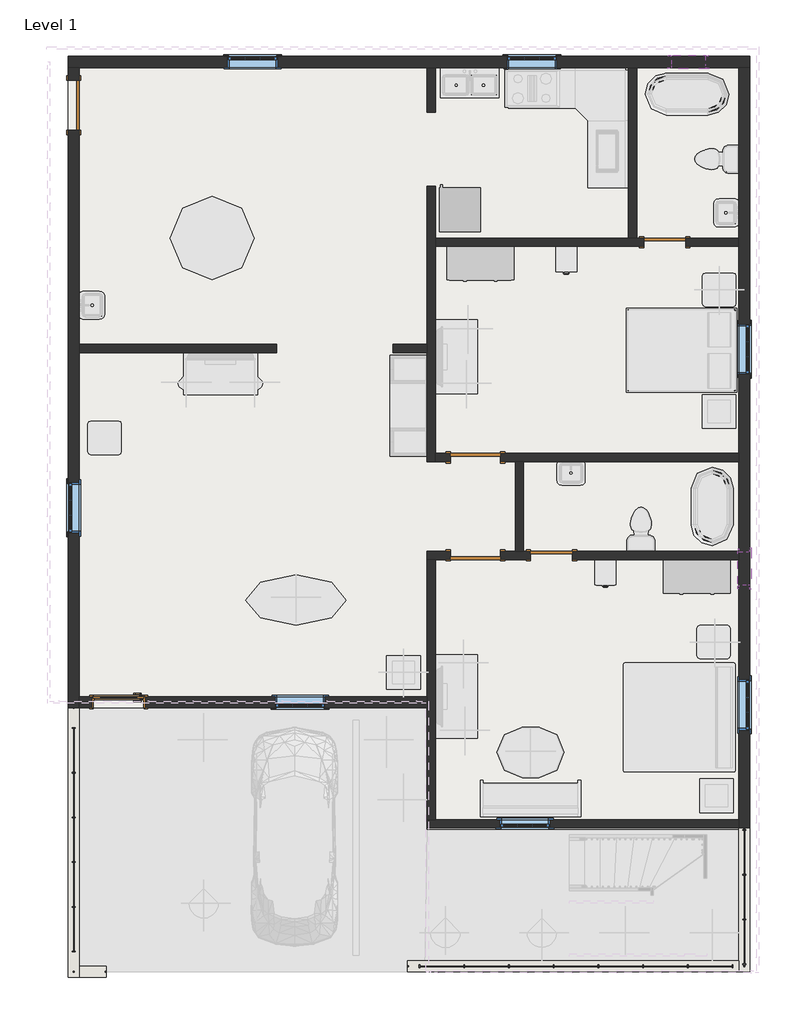
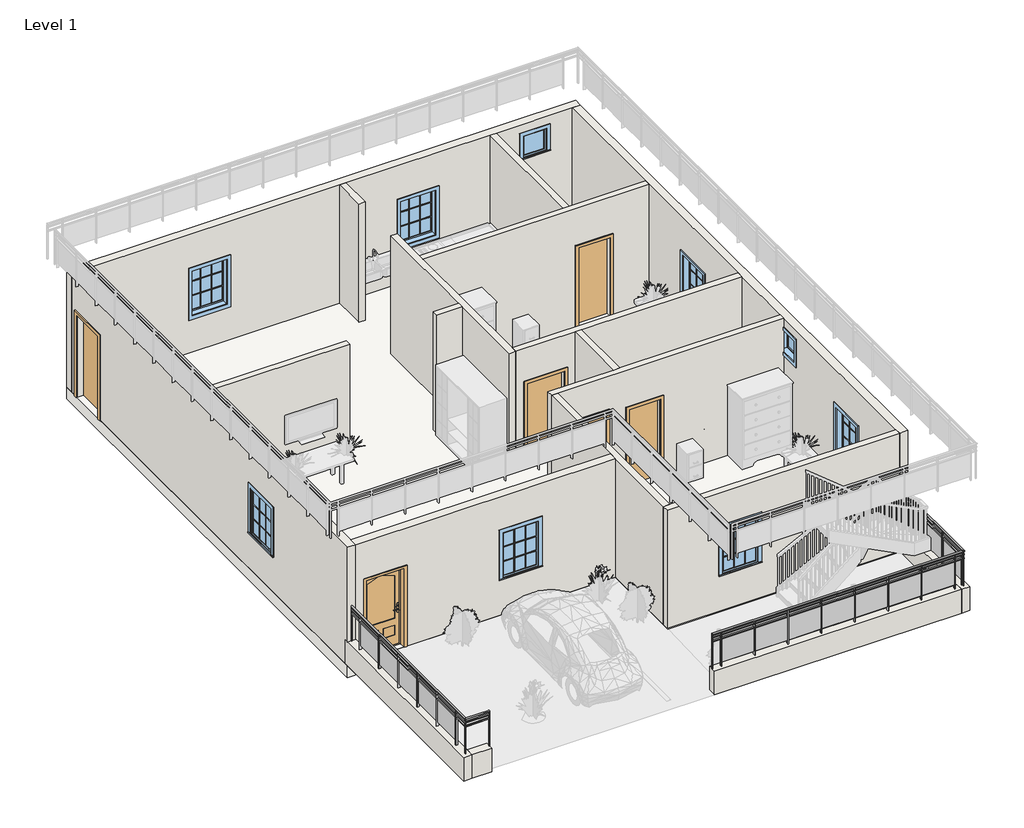
# One storey, part 1 of 5: 19 walls, 9 windows, 6 doors, 2 railings, 1 slab.
"""IFC4 building model written with IfcOpenShell, lengths in millimetres."""

from ifc_helpers import new_model, si_unit, frame, origin, origin_with_axes, place, context, project, spatial, polyline, circle_curve, ellipse_curve, outline, extrude, faceted_brep, transform, mapped, element, save
from ifc_brep_helpers import plane_surface, cylinder_surface, advanced_brep
from components import door_1768e003, door_255cab33, door_719f80de, door_16372e1c, door_686f89d2, window_29c06734, window_5c190c7e, window_e41d21a6

model = new_model("IFC4")

# Units and contexts
model_context = context("Model", 3, world=origin())
ifc_project = project(units=[si_unit("LENGTHUNIT", "METRE", prefix="MILLI")], contexts=[model_context])

# Site, building, storey
site = spatial("IfcSite", under=ifc_project)
building = spatial("IfcBuilding", under=site)
storey = spatial("IfcBuildingStorey", under=building, Name="Level 1", Elevation=0.0)

# Doors
placement = place(None, origin())
door_shape = door_1768e003(model_context)
element("IfcDoor", 1, ObjectType="36\" x 80\"", at=placement, inside=storey, context=model_context, shape_type="MappedRepresentation", body=[
    mapped(door_shape, transform((-11404.4241134, 2269.2383056, 0.0), x_axis=(1.0, 0.0, 0.0), y_axis=(0.0, 1.0, 0.0), z_axis=(0.0, 0.0, 1.0))),
])
door_2_shape = door_255cab33(model_context)
element("IfcDoor", 2, ObjectType="Single-Flush : 30\" x 80\"", at=placement, inside=storey, context=model_context, shape_type="MappedRepresentation", body=[
    mapped(door_2_shape, transform((-3530.4241134, 4933.0633056, 0.0), x_axis=(-1.0, 0.0, 0.0), y_axis=(0.0, -1.0, 0.0), z_axis=(0.0, 0.0, 1.0))),
])
element("IfcDoor", 3, ObjectType="Single-Flush : 30\" x 80\"", at=placement, inside=storey, context=model_context, shape_type="MappedRepresentation", body=[
    mapped(door_2_shape, transform((-1473.0241134, 10622.6633056, 0.0), x_axis=(-1.0, 0.0, 0.0), y_axis=(0.0, -1.0, 0.0), z_axis=(0.0, 0.0, 1.0))),
])
door_3_shape = door_719f80de(model_context)
element("IfcDoor", 4, ObjectType="Single-Flush : 36\" x 84\"", at=placement, inside=storey, context=model_context, shape_type="MappedRepresentation", body=[
    mapped(door_3_shape, transform((-12217.2241134, 13111.8633056, 0.0), x_axis=(0.0, 1.0, 0.0), y_axis=(-1.0, 0.0, 0.0), z_axis=(0.0, 0.0, 1.0))),
])
door_4_shape = door_16372e1c(model_context)
element("IfcDoor", 5, ObjectType="Single-Flush : 36\" x 84\"", at=placement, inside=storey, context=model_context, shape_type="MappedRepresentation", body=[
    mapped(door_4_shape, transform((-4914.7241134, 4933.0633056, 0.0), x_axis=(-1.0, 0.0, 0.0), y_axis=(0.0, -1.0, 0.0), z_axis=(0.0, 0.0, 1.0))),
])
door_5_shape = door_686f89d2(model_context)
element("IfcDoor", 6, ObjectType="Single-Flush : 36\" x 84\"", at=placement, inside=storey, context=model_context, shape_type="MappedRepresentation", body=[
    mapped(door_5_shape, transform((-4914.7241134, 6711.0633056, 0.0), x_axis=(-1.0, 0.0, 0.0), y_axis=(0.0, -1.0, 0.0), z_axis=(0.0, 0.0, 1.0))),
])

# Railings
element("IfcRailing", 7, ObjectType="Glass Panel - Bottom Fill", at=placement, inside=storey, context=model_context, shape_type="SolidModel", body=[
    advanced_brep(
    [(-12236.2741134, 2164.4633056, 1504.95), (-12198.1741134, 2164.4633056, 1504.95), (-11633.0241134, -2655.1866944, 1504.95), (-11633.0241134, -2617.0866944, 1504.95), (-12236.2741134, -2655.1866944, 1504.95), (-12198.1741134, -2617.0866944, 1504.95)],
    [
        (0, 1, circle_curve(frame((-12217.2241134, 2164.4633056, 1504.95), z_axis=(0.0, 1.0, 0.0), x_axis=(1.0, 0.0, 0.0)), 19.05)),
        (1, 0, circle_curve(frame((-12217.2241134, 2164.4633056, 1504.95), z_axis=(0.0, 1.0, 0.0), x_axis=(1.0, 0.0, 0.0)), 19.05)),
        (2, 3, circle_curve(frame((-11633.0241134, -2636.1366944, 1504.95), z_axis=(1.0, 0.0, 0.0), x_axis=(0.0, 1.0, 0.0)), 19.05)),
        (3, 2, circle_curve(frame((-11633.0241134, -2636.1366944, 1504.95), z_axis=(1.0, 0.0, 0.0), x_axis=(0.0, 1.0, 0.0)), 19.05)),
        (0, 4),
        (4, 5, ellipse_curve(frame((-12217.2241134, -2636.1366944, 1504.95), z_axis=(-0.707106781186546, 0.7071067811865491, 0.0), x_axis=(0.7071067811865492, 0.7071067811865458, 0.0)), 26.9407684, 19.05)),
        (5, 1),
        (5, 4, ellipse_curve(frame((-12217.2241134, -2636.1366944, 1504.95), z_axis=(-0.707106781186546, 0.7071067811865491, 0.0), x_axis=(0.7071067811865492, 0.7071067811865458, 0.0)), 26.9407684, 19.05)),
        (4, 2),
        (3, 5),
    ],
    [
        plane_surface(frame((-12217.2241134, 2164.4633056, 1524.0), z_axis=(0.0, 1.0, 0.0), x_axis=(0.0, 0.0, -1.0))),
        plane_surface(frame((-11633.0241134, -2636.1366944, 1524.0), z_axis=(1.0, 0.0, 0.0), x_axis=(0.0, 1.0, 0.0))),
        cylinder_surface(frame((-12217.2241134, 2164.4633056, 1504.95), z_axis=(0.0, 1.0, 0.0), x_axis=(1.0, 0.0, 0.0)), 19.05),
        cylinder_surface(frame((-12217.2241134, -2636.1366944, 1504.95), z_axis=(-1.0, 0.0, 0.0), x_axis=(0.0, 1.0, 0.0)), 19.05),
    ],
    [
        (0, [[1, 2]]),
        (1, [[3, 4]]),
        (2, [[-1, 5, 6, 7]]),
        (2, [[-2, -7, 8, -5]]),
        (3, [[-6, 9, -4, 10]]),
        (3, [[-8, -10, -3, -9]]),
    ],
),
    faceted_brep([(-12229.9241134, 2164.4633056, 1435.1), (-12204.5241134, 2164.4633056, 1435.1), (-12204.5241134, 2164.4633056, 1409.7), (-12229.9241134, 2164.4633056, 1409.7), (-12229.9241134, -2648.8366944, 1435.1), (-12204.5241134, -2623.4366944, 1435.1), (-12204.5241134, -2623.4366944, 1409.7), (-12229.9241134, -2648.8366944, 1409.7), (-11633.0241134, -2648.8366944, 1435.1), (-11633.0241134, -2648.8366944, 1409.7), (-11633.0241134, -2623.4366944, 1409.7), (-11633.0241134, -2623.4366944, 1435.1)], [[[0, 1, 2, 3]], [[1, 0, 4, 5]], [[2, 1, 5, 6]], [[3, 2, 6, 7]], [[0, 3, 7, 4]], [[8, 9, 10, 11]], [[5, 4, 8, 11]], [[6, 5, 11, 10]], [[7, 6, 10, 9]], [[4, 7, 9, 8]]]),
    faceted_brep([(-12229.9241134, 2164.4633056, 1333.5), (-12204.5241134, 2164.4633056, 1333.5), (-12204.5241134, 2164.4633056, 1308.1), (-12229.9241134, 2164.4633056, 1308.1), (-12229.9241134, -2648.8366944, 1333.5), (-12204.5241134, -2623.4366944, 1333.5), (-12204.5241134, -2623.4366944, 1308.1), (-12229.9241134, -2648.8366944, 1308.1), (-11633.0241134, -2648.8366944, 1333.5), (-11633.0241134, -2648.8366944, 1308.1), (-11633.0241134, -2623.4366944, 1308.1), (-11633.0241134, -2623.4366944, 1333.5)], [[[0, 1, 2, 3]], [[1, 0, 4, 5]], [[2, 1, 5, 6]], [[3, 2, 6, 7]], [[0, 3, 7, 4]], [[8, 9, 10, 11]], [[5, 4, 8, 11]], [[6, 5, 11, 10]], [[7, 6, 10, 9]], [[4, 7, 9, 8]]]),
    extrude(outline(polyline([(-12242.6241134, -2261.4866944), (-12191.8241134, -2261.4866944), (-12191.8241134, -2274.1866944), (-12242.6241134, -2274.1866944), (-12242.6241134, -2261.4866944)])), frame((0.0, 0.0, 609.6), z_axis=(0.0, 0.0, 1.0), x_axis=(1.0, 0.0, 0.0)), (0.0, 0.0, 1.0), 876.3),
    extrude(outline(polyline([(-12210.6889564, -1455.0366944), (-12210.6889564, -2267.8366944), (-12217.0389564, -2267.8366944), (-12217.0389564, -1455.0366944), (-12210.6889564, -1455.0366944)])), frame((0.0, 0.0, 711.2), z_axis=(0.0, 0.0, 1.0), x_axis=(1.0, 0.0, 0.0)), (0.0, 0.0, 1.0), 596.9),
    extrude(outline(polyline([(-12242.6241134, -1448.6866944), (-12191.8241134, -1448.6866944), (-12191.8241134, -1461.3866944), (-12242.6241134, -1461.3866944), (-12242.6241134, -1448.6866944)])), frame((0.0, 0.0, 609.6), z_axis=(0.0, 0.0, 1.0), x_axis=(1.0, 0.0, 0.0)), (0.0, 0.0, 1.0), 876.3),
    extrude(outline(polyline([(-12210.6889564, -642.2366944), (-12210.6889564, -1455.0366944), (-12217.0389564, -1455.0366944), (-12217.0389564, -642.2366944), (-12210.6889564, -642.2366944)])), frame((0.0, 0.0, 711.2), z_axis=(0.0, 0.0, 1.0), x_axis=(1.0, 0.0, 0.0)), (0.0, 0.0, 1.0), 596.9),
    extrude(outline(polyline([(-12242.6241134, -635.8866944), (-12191.8241134, -635.8866944), (-12191.8241134, -648.5866944), (-12242.6241134, -648.5866944), (-12242.6241134, -635.8866944)])), frame((0.0, 0.0, 609.6), z_axis=(0.0, 0.0, 1.0), x_axis=(1.0, 0.0, 0.0)), (0.0, 0.0, 1.0), 876.3),
    extrude(outline(polyline([(-12210.6889564, 170.5633056), (-12210.6889564, -642.2366944), (-12217.0389564, -642.2366944), (-12217.0389564, 170.5633056), (-12210.6889564, 170.5633056)])), frame((0.0, 0.0, 711.2), z_axis=(0.0, 0.0, 1.0), x_axis=(1.0, 0.0, 0.0)), (0.0, 0.0, 1.0), 596.9),
    extrude(outline(polyline([(-12242.6241134, 176.9133056), (-12191.8241134, 176.9133056), (-12191.8241134, 164.2133056), (-12242.6241134, 164.2133056), (-12242.6241134, 176.9133056)])), frame((0.0, 0.0, 609.6), z_axis=(0.0, 0.0, 1.0), x_axis=(1.0, 0.0, 0.0)), (0.0, 0.0, 1.0), 876.3),
    extrude(outline(polyline([(-12210.6889564, 983.3633056), (-12210.6889564, 170.5633056), (-12217.0389564, 170.5633056), (-12217.0389564, 983.3633056), (-12210.6889564, 983.3633056)])), frame((0.0, 0.0, 711.2), z_axis=(0.0, 0.0, 1.0), x_axis=(1.0, 0.0, 0.0)), (0.0, 0.0, 1.0), 596.9),
    extrude(outline(polyline([(-12242.6241134, 989.7133056), (-12191.8241134, 989.7133056), (-12191.8241134, 977.0133056), (-12242.6241134, 977.0133056), (-12242.6241134, 989.7133056)])), frame((0.0, 0.0, 609.6), z_axis=(0.0, 0.0, 1.0), x_axis=(1.0, 0.0, 0.0)), (0.0, 0.0, 1.0), 876.3),
    extrude(outline(polyline([(-12210.6889564, 1796.1633056), (-12210.6889564, 983.3633056), (-12217.0389564, 983.3633056), (-12217.0389564, 1796.1633056), (-12210.6889564, 1796.1633056)])), frame((0.0, 0.0, 711.2), z_axis=(0.0, 0.0, 1.0), x_axis=(1.0, 0.0, 0.0)), (0.0, 0.0, 1.0), 596.9),
    extrude(outline(polyline([(-12242.6241134, 1802.5133056), (-12191.8241134, 1802.5133056), (-12191.8241134, 1789.8133056), (-12242.6241134, 1789.8133056), (-12242.6241134, 1802.5133056)])), frame((0.0, 0.0, 609.6), z_axis=(0.0, 0.0, 1.0), x_axis=(1.0, 0.0, 0.0)), (0.0, 0.0, 1.0), 876.3),
    extrude(outline(polyline([(-12226.7491134, -2626.6116944), (-12207.6991134, -2626.6116944), (-12207.6991134, -2645.6616944), (-12226.7491134, -2645.6616944), (-12226.7491134, -2626.6116944)])), frame((0.0, 0.0, 609.6), z_axis=(0.0, 0.0, 1.0), x_axis=(1.0, 0.0, 0.0)), (0.0, 0.0, 1.0), 876.3),
    extrude(outline(polyline([(-11645.7241134, -2645.6616944), (-11645.7241134, -2626.6116944), (-11626.6741134, -2626.6116944), (-11626.6741134, -2645.6616944), (-11645.7241134, -2645.6616944)])), frame((0.0, 0.0, 609.6), z_axis=(0.0, 0.0, 1.0), x_axis=(1.0, 0.0, 0.0)), (0.0, 0.0, 1.0), 876.3),
    extrude(outline(polyline([(-12226.7491134, 2170.8133056), (-12207.6991134, 2170.8133056), (-12207.6991134, 2151.7633056), (-12226.7491134, 2151.7633056), (-12226.7491134, 2170.8133056)])), frame((0.0, 0.0, 609.6), z_axis=(0.0, 0.0, 1.0), x_axis=(1.0, 0.0, 0.0)), (0.0, 0.0, 1.0), 876.3),
])
element("IfcRailing", 8, ObjectType="Glass Panel - Bottom Fill", at=placement, inside=storey, context=model_context, shape_type="SolidModel", body=[
    advanced_brep(
    [(-44.2741134, -19.9366944, 1504.95), (-6.1741134, -19.9366944, 1504.95), (-6146.6241134, -2515.4866944, 1504.95), (-6146.6241134, -2553.5866944, 1504.95), (-44.2741134, -2515.4866944, 1504.95), (-6.1741134, -2553.5866944, 1504.95)],
    [
        (0, 1, circle_curve(frame((-25.2241134, -19.9366944, 1504.95), z_axis=(0.0, 1.0, 0.0), x_axis=(1.0, 0.0, 0.0)), 19.05)),
        (1, 0, circle_curve(frame((-25.2241134, -19.9366944, 1504.95), z_axis=(0.0, 1.0, 0.0), x_axis=(1.0, 0.0, 0.0)), 19.05)),
        (2, 3, circle_curve(frame((-6146.6241134, -2534.5366944, 1504.95), z_axis=(-1.0, 0.0, 0.0), x_axis=(0.0, -1.0, 0.0)), 19.05)),
        (3, 2, circle_curve(frame((-6146.6241134, -2534.5366944, 1504.95), z_axis=(-1.0, 0.0, 0.0), x_axis=(0.0, -1.0, 0.0)), 19.05)),
        (0, 4),
        (4, 5, ellipse_curve(frame((-25.2241134, -2534.5366944, 1504.95), z_axis=(0.7071067811865492, 0.7071067811865458, 0.0), x_axis=(-0.7071067811865457, 0.7071067811865492, 0.0)), 26.9407684, 19.05)),
        (5, 1),
        (5, 4, ellipse_curve(frame((-25.2241134, -2534.5366944, 1504.95), z_axis=(0.7071067811865492, 0.7071067811865458, 0.0), x_axis=(-0.7071067811865457, 0.7071067811865492, 0.0)), 26.9407684, 19.05)),
        (4, 2),
        (3, 5),
    ],
    [
        plane_surface(frame((-25.2241134, -19.9366944, 1524.0), z_axis=(0.0, 1.0, 0.0), x_axis=(0.0, 0.0, -1.0))),
        plane_surface(frame((-6146.6241134, -2534.5366944, 1524.0), z_axis=(-1.0, 0.0, 0.0), x_axis=(0.0, -1.0, 0.0))),
        cylinder_surface(frame((-25.2241134, -19.9366944, 1504.95), z_axis=(0.0, 1.0, 0.0), x_axis=(1.0, 0.0, 0.0)), 19.05),
        cylinder_surface(frame((-25.2241134, -2534.5366944, 1504.95), z_axis=(1.0, 0.0, 0.0), x_axis=(0.0, -1.0, 0.0)), 19.05),
    ],
    [
        (0, [[1, 2]]),
        (1, [[3, 4]]),
        (2, [[-1, 5, 6, 7]]),
        (2, [[-2, -7, 8, -5]]),
        (3, [[-6, 9, -4, 10]]),
        (3, [[-8, -10, -3, -9]]),
    ],
),
    faceted_brep([(-37.9241134, -19.9366944, 1435.1), (-12.5241134, -19.9366944, 1435.1), (-12.5241134, -19.9366944, 1409.7), (-37.9241134, -19.9366944, 1409.7), (-37.9241134, -2521.8366944, 1435.1), (-12.5241134, -2547.2366944, 1435.1), (-12.5241134, -2547.2366944, 1409.7), (-37.9241134, -2521.8366944, 1409.7), (-6146.6241134, -2521.8366944, 1435.1), (-6146.6241134, -2521.8366944, 1409.7), (-6146.6241134, -2547.2366944, 1409.7), (-6146.6241134, -2547.2366944, 1435.1)], [[[0, 1, 2, 3]], [[1, 0, 4, 5]], [[2, 1, 5, 6]], [[3, 2, 6, 7]], [[0, 3, 7, 4]], [[8, 9, 10, 11]], [[5, 4, 8, 11]], [[6, 5, 11, 10]], [[7, 6, 10, 9]], [[4, 7, 9, 8]]]),
    faceted_brep([(-37.9241134, -19.9366944, 1333.5), (-12.5241134, -19.9366944, 1333.5), (-12.5241134, -19.9366944, 1308.1), (-37.9241134, -19.9366944, 1308.1), (-37.9241134, -2521.8366944, 1333.5), (-12.5241134, -2547.2366944, 1333.5), (-12.5241134, -2547.2366944, 1308.1), (-37.9241134, -2521.8366944, 1308.1), (-6146.6241134, -2521.8366944, 1333.5), (-6146.6241134, -2521.8366944, 1308.1), (-6146.6241134, -2547.2366944, 1308.1), (-6146.6241134, -2547.2366944, 1333.5)], [[[0, 1, 2, 3]], [[1, 0, 4, 5]], [[2, 1, 5, 6]], [[3, 2, 6, 7]], [[0, 3, 7, 4]], [[8, 9, 10, 11]], [[5, 4, 8, 11]], [[6, 5, 11, 10]], [[7, 6, 10, 9]], [[4, 7, 9, 8]]]),
    extrude(outline(polyline([(-5924.3741134, -2509.1366944), (-5924.3741134, -2559.9366944), (-5937.0741134, -2559.9366944), (-5937.0741134, -2509.1366944), (-5924.3741134, -2509.1366944)])), frame((0.0, 0.0, 609.6), z_axis=(0.0, 0.0, 1.0), x_axis=(1.0, 0.0, 0.0)), (0.0, 0.0, 1.0), 876.3),
    extrude(outline(polyline([(-5117.9241134, -2541.0718514), (-5930.7241134, -2541.0718514), (-5930.7241134, -2534.7218514), (-5117.9241134, -2534.7218514), (-5117.9241134, -2541.0718514)])), frame((0.0, 0.0, 711.2), z_axis=(0.0, 0.0, 1.0), x_axis=(1.0, 0.0, 0.0)), (0.0, 0.0, 1.0), 596.9),
    extrude(outline(polyline([(-5111.5741134, -2509.1366944), (-5111.5741134, -2559.9366944), (-5124.2741134, -2559.9366944), (-5124.2741134, -2509.1366944), (-5111.5741134, -2509.1366944)])), frame((0.0, 0.0, 609.6), z_axis=(0.0, 0.0, 1.0), x_axis=(1.0, 0.0, 0.0)), (0.0, 0.0, 1.0), 876.3),
    extrude(outline(polyline([(-4305.1241134, -2541.0718514), (-5117.9241134, -2541.0718514), (-5117.9241134, -2534.7218514), (-4305.1241134, -2534.7218514), (-4305.1241134, -2541.0718514)])), frame((0.0, 0.0, 711.2), z_axis=(0.0, 0.0, 1.0), x_axis=(1.0, 0.0, 0.0)), (0.0, 0.0, 1.0), 596.9),
    extrude(outline(polyline([(-4298.7741134, -2509.1366944), (-4298.7741134, -2559.9366944), (-4311.4741134, -2559.9366944), (-4311.4741134, -2509.1366944), (-4298.7741134, -2509.1366944)])), frame((0.0, 0.0, 609.6), z_axis=(0.0, 0.0, 1.0), x_axis=(1.0, 0.0, 0.0)), (0.0, 0.0, 1.0), 876.3),
    extrude(outline(polyline([(-3492.3241134, -2541.0718514), (-4305.1241134, -2541.0718514), (-4305.1241134, -2534.7218514), (-3492.3241134, -2534.7218514), (-3492.3241134, -2541.0718514)])), frame((0.0, 0.0, 711.2), z_axis=(0.0, 0.0, 1.0), x_axis=(1.0, 0.0, 0.0)), (0.0, 0.0, 1.0), 596.9),
    extrude(outline(polyline([(-3485.9741134, -2509.1366944), (-3485.9741134, -2559.9366944), (-3498.6741134, -2559.9366944), (-3498.6741134, -2509.1366944), (-3485.9741134, -2509.1366944)])), frame((0.0, 0.0, 609.6), z_axis=(0.0, 0.0, 1.0), x_axis=(1.0, 0.0, 0.0)), (0.0, 0.0, 1.0), 876.3),
    extrude(outline(polyline([(-2679.5241134, -2541.0718514), (-3492.3241134, -2541.0718514), (-3492.3241134, -2534.7218514), (-2679.5241134, -2534.7218514), (-2679.5241134, -2541.0718514)])), frame((0.0, 0.0, 711.2), z_axis=(0.0, 0.0, 1.0), x_axis=(1.0, 0.0, 0.0)), (0.0, 0.0, 1.0), 596.9),
    extrude(outline(polyline([(-2673.1741134, -2509.1366944), (-2673.1741134, -2559.9366944), (-2685.8741134, -2559.9366944), (-2685.8741134, -2509.1366944), (-2673.1741134, -2509.1366944)])), frame((0.0, 0.0, 609.6), z_axis=(0.0, 0.0, 1.0), x_axis=(1.0, 0.0, 0.0)), (0.0, 0.0, 1.0), 876.3),
    extrude(outline(polyline([(-1866.7241134, -2541.0718514), (-2679.5241134, -2541.0718514), (-2679.5241134, -2534.7218514), (-1866.7241134, -2534.7218514), (-1866.7241134, -2541.0718514)])), frame((0.0, 0.0, 711.2), z_axis=(0.0, 0.0, 1.0), x_axis=(1.0, 0.0, 0.0)), (0.0, 0.0, 1.0), 596.9),
    extrude(outline(polyline([(-1860.3741134, -2509.1366944), (-1860.3741134, -2559.9366944), (-1873.0741134, -2559.9366944), (-1873.0741134, -2509.1366944), (-1860.3741134, -2509.1366944)])), frame((0.0, 0.0, 609.6), z_axis=(0.0, 0.0, 1.0), x_axis=(1.0, 0.0, 0.0)), (0.0, 0.0, 1.0), 876.3),
    extrude(outline(polyline([(-1053.9241134, -2541.0718514), (-1866.7241134, -2541.0718514), (-1866.7241134, -2534.7218514), (-1053.9241134, -2534.7218514), (-1053.9241134, -2541.0718514)])), frame((0.0, 0.0, 711.2), z_axis=(0.0, 0.0, 1.0), x_axis=(1.0, 0.0, 0.0)), (0.0, 0.0, 1.0), 596.9),
    extrude(outline(polyline([(-1047.5741134, -2509.1366944), (-1047.5741134, -2559.9366944), (-1060.2741134, -2559.9366944), (-1060.2741134, -2509.1366944), (-1047.5741134, -2509.1366944)])), frame((0.0, 0.0, 609.6), z_axis=(0.0, 0.0, 1.0), x_axis=(1.0, 0.0, 0.0)), (0.0, 0.0, 1.0), 876.3),
    extrude(outline(polyline([(-241.1241134, -2541.0718514), (-1053.9241134, -2541.0718514), (-1053.9241134, -2534.7218514), (-241.1241134, -2534.7218514), (-241.1241134, -2541.0718514)])), frame((0.0, 0.0, 711.2), z_axis=(0.0, 0.0, 1.0), x_axis=(1.0, 0.0, 0.0)), (0.0, 0.0, 1.0), 596.9),
    extrude(outline(polyline([(-234.7741134, -2509.1366944), (-234.7741134, -2559.9366944), (-247.4741134, -2559.9366944), (-247.4741134, -2509.1366944), (-234.7741134, -2509.1366944)])), frame((0.0, 0.0, 609.6), z_axis=(0.0, 0.0, 1.0), x_axis=(1.0, 0.0, 0.0)), (0.0, 0.0, 1.0), 876.3),
    extrude(outline(polyline([(-50.6241134, -2490.0866944), (0.1758866, -2490.0866944), (0.1758866, -2502.7866944), (-50.6241134, -2502.7866944), (-50.6241134, -2490.0866944)])), frame((0.0, 0.0, 609.6), z_axis=(0.0, 0.0, 1.0), x_axis=(1.0, 0.0, 0.0)), (0.0, 0.0, 1.0), 876.3),
    extrude(outline(polyline([(-18.6889564, -1683.6366944), (-18.6889564, -2496.4366944), (-25.0389564, -2496.4366944), (-25.0389564, -1683.6366944), (-18.6889564, -1683.6366944)])), frame((0.0, 0.0, 711.2), z_axis=(0.0, 0.0, 1.0), x_axis=(1.0, 0.0, 0.0)), (0.0, 0.0, 1.0), 596.9),
    extrude(outline(polyline([(-50.6241134, -1677.2866944), (0.1758866, -1677.2866944), (0.1758866, -1689.9866944), (-50.6241134, -1689.9866944), (-50.6241134, -1677.2866944)])), frame((0.0, 0.0, 609.6), z_axis=(0.0, 0.0, 1.0), x_axis=(1.0, 0.0, 0.0)), (0.0, 0.0, 1.0), 876.3),
    extrude(outline(polyline([(-18.6889564, -870.8366944), (-18.6889564, -1683.6366944), (-25.0389564, -1683.6366944), (-25.0389564, -870.8366944), (-18.6889564, -870.8366944)])), frame((0.0, 0.0, 711.2), z_axis=(0.0, 0.0, 1.0), x_axis=(1.0, 0.0, 0.0)), (0.0, 0.0, 1.0), 596.9),
    extrude(outline(polyline([(-50.6241134, -864.4866944), (0.1758866, -864.4866944), (0.1758866, -877.1866944), (-50.6241134, -877.1866944), (-50.6241134, -864.4866944)])), frame((0.0, 0.0, 609.6), z_axis=(0.0, 0.0, 1.0), x_axis=(1.0, 0.0, 0.0)), (0.0, 0.0, 1.0), 876.3),
    extrude(outline(polyline([(-18.6889564, -58.0366944), (-18.6889564, -870.8366944), (-25.0389564, -870.8366944), (-25.0389564, -58.0366944), (-18.6889564, -58.0366944)])), frame((0.0, 0.0, 711.2), z_axis=(0.0, 0.0, 1.0), x_axis=(1.0, 0.0, 0.0)), (0.0, 0.0, 1.0), 596.9),
    extrude(outline(polyline([(-50.6241134, -51.6866944), (0.1758866, -51.6866944), (0.1758866, -64.3866944), (-50.6241134, -64.3866944), (-50.6241134, -51.6866944)])), frame((0.0, 0.0, 609.6), z_axis=(0.0, 0.0, 1.0), x_axis=(1.0, 0.0, 0.0)), (0.0, 0.0, 1.0), 876.3),
    extrude(outline(polyline([(-34.7491134, -2525.0116944), (-15.6991134, -2525.0116944), (-15.6991134, -2544.0616944), (-34.7491134, -2544.0616944), (-34.7491134, -2525.0116944)])), frame((0.0, 0.0, 609.6), z_axis=(0.0, 0.0, 1.0), x_axis=(1.0, 0.0, 0.0)), (0.0, 0.0, 1.0), 876.3),
    extrude(outline(polyline([(-6133.9241134, -2525.0116944), (-6133.9241134, -2544.0616944), (-6152.9741134, -2544.0616944), (-6152.9741134, -2525.0116944), (-6133.9241134, -2525.0116944)])), frame((0.0, 0.0, 609.6), z_axis=(0.0, 0.0, 1.0), x_axis=(1.0, 0.0, 0.0)), (0.0, 0.0, 1.0), 876.3),
    extrude(outline(polyline([(-34.7491134, -13.5866944), (-15.6991134, -13.5866944), (-15.6991134, -32.6366944), (-34.7491134, -32.6366944), (-34.7491134, -13.5866944)])), frame((0.0, 0.0, 609.6), z_axis=(0.0, 0.0, 1.0), x_axis=(1.0, 0.0, 0.0)), (0.0, 0.0, 1.0), 876.3),
])

# Slab
element("IfcSlab", 9, ObjectType="Generic - 12\"", at=placement, inside=storey, context=model_context, shape_type="SweptSolid", body=[
    extrude(outline(polyline([(76.3758866, 14000.8633056), (76.3758866, -45.3366944), (-5791.0241134, -45.3366944), (-5791.0241134, 2164.4633056), (-12318.8241134, 2164.4633056), (-12318.8241134, 14000.8633056), (76.3758866, 14000.8633056)])), frame((0.0, 0.0, -304.8), z_axis=(0.0, 0.0, 1.0), x_axis=(1.0, 0.0, 0.0)), (0.0, 0.0, 1.0), 304.8),
])

# Walls
element("IfcWall", 10, ObjectType="Generic - 2'", at=placement, inside=storey, context=model_context, shape_type="SweptSolid", body=[
    extrude(outline(polyline([(-6146.6241134, -2432.9366944), (-126.8241134, -2432.9366944), (-126.8241134, -2636.1366944), (-6146.6241134, -2636.1366944), (-6146.6241134, -2432.9366944)])), origin_with_axes(), (0.0, 0.0, 1.0), 609.6),
])
element("IfcWall", 11, ObjectType="Generic - 2'", at=placement, inside=storey, context=model_context, shape_type="Brep", body=[
    faceted_brep([(-12115.6241134, -2737.7366944, 0.0), (-12115.6241134, -2534.5366944, 0.0), (-12115.6241134, 2164.4633056, 0.0), (-12115.6241134, 2266.0633056, 0.0), (-12115.6241134, 2266.0633056, 609.6), (-12115.6241134, -2534.5366944, 609.6), (-12115.6241134, -2737.7366944, 609.6), (-12318.8241134, -2737.7366944, 0.0), (-12318.8241134, -2737.7366944, 609.6), (-12318.8241134, 2266.0633056, 609.6), (-12318.8241134, 2266.0633056, 0.0)], [[[0, 1, 2, 3, 4, 5, 6]], [[7, 8, 9, 10]], [[3, 2, 1, 0, 7, 10]], [[4, 3, 10, 9]], [[6, 5, 4, 9, 8]], [[0, 6, 8, 7]]]),
])
element("IfcWall", 12, ObjectType="Generic - 2'", at=placement, inside=storey, context=model_context, shape_type="Brep", body=[
    faceted_brep([(-126.8241134, 56.2633056, 0.0), (-126.8241134, -19.9366944, 0.0), (-126.8241134, -2432.9366944, 0.0), (-126.8241134, -2636.1366944, 0.0), (-126.8241134, -2636.1366944, 609.6), (-126.8241134, -2432.9366944, 609.6), (-126.8241134, 56.2633056, 609.6), (76.3758866, 56.2633056, 0.0), (76.3758866, 56.2633056, 609.6), (76.3758866, -2636.1366944, 609.6), (76.3758866, -2636.1366944, 0.0)], [[[0, 1, 2, 3, 4, 5, 6]], [[7, 8, 9, 10]], [[3, 2, 1, 0, 7, 10]], [[6, 5, 4, 9, 8]], [[0, 6, 8, 7]], [[4, 3, 10, 9]]]),
])
element("IfcWall", 13, ObjectType="Generic - 2'", at=placement, inside=storey, context=model_context, shape_type="SweptSolid", body=[
    extrude(outline(polyline([(-11633.0241134, -2737.7366944), (-12115.6241134, -2737.7366944), (-12115.6241134, -2534.5366944), (-11633.0241134, -2534.5366944), (-11633.0241134, -2737.7366944)])), origin_with_axes(), (0.0, 0.0, 1.0), 609.6),
])
element("IfcWall", 14, ObjectType="Generic - 8\"", at=placement, inside=storey, context=model_context, shape_type="Brep", body=[
    faceted_brep([(-12318.8241134, 13797.6633056, 0.0), (-12115.6241134, 13797.6633056, 0.0), (-5791.0241134, 13797.6633056, 0.0), (-5638.6241134, 13797.6633056, 0.0), (-2133.4241134, 13797.6633056, 0.0), (-1981.0241134, 13797.6633056, 0.0), (-126.8241134, 13797.6633056, 0.0), (76.3758866, 13797.6633056, 0.0), (76.3758866, 13797.6633056, 3048.0), (-126.8241134, 13797.6633056, 3048.0), (-1981.0241134, 13797.6633056, 3048.0), (-2133.4241134, 13797.6633056, 3048.0), (-5638.6241134, 13797.6633056, 3048.0), (-5791.0241134, 13797.6633056, 3048.0), (-12115.6241134, 13797.6633056, 3048.0), (-12318.8241134, 13797.6633056, 3048.0), (-8508.8241134, 13797.6633056, 2133.6), (-8508.8241134, 13797.6633056, 914.4), (-9423.2241134, 13797.6633056, 914.4), (-9423.2241134, 13797.6633056, 2133.6), (-3428.8241134, 13797.6633056, 2133.6), (-3428.8241134, 13797.6633056, 914.4), (-4343.2241134, 13797.6633056, 914.4), (-4343.2241134, 13797.6633056, 2133.6), (-1346.0241134, 13797.6633056, 2768.6), (-736.4241134, 13797.6633056, 2768.6), (-736.4241134, 13797.6633056, 2159.0), (-1346.0241134, 13797.6633056, 2159.0), (-12318.8241134, 14000.8633056, 0.0), (-12318.8241134, 14000.8633056, 3048.0), (76.3758866, 14000.8633056, 3048.0), (76.3758866, 14000.8633056, 0.0), (-8508.8241134, 14000.8633056, 2133.6), (-9423.2241134, 14000.8633056, 2133.6), (-9423.2241134, 14000.8633056, 914.4), (-8508.8241134, 14000.8633056, 914.4), (-3428.8241134, 14000.8633056, 2133.6), (-4343.2241134, 14000.8633056, 2133.6), (-4343.2241134, 14000.8633056, 914.4), (-3428.8241134, 14000.8633056, 914.4), (-1346.0241134, 14000.8633056, 2768.6), (-1346.0241134, 14000.8633056, 2159.0), (-736.4241134, 14000.8633056, 2159.0), (-736.4241134, 14000.8633056, 2768.6)], [[[0, 1, 2, 3, 4, 5, 6, 7, 8, 9, 10, 11, 12, 13, 14, 15], [16, 17, 18, 19], [20, 21, 22, 23], [24, 25, 26, 27]], [[28, 29, 30, 31], [32, 33, 34, 35], [36, 37, 38, 39], [40, 41, 42, 43]], [[7, 6, 5, 4, 3, 2, 1, 0, 28, 31]], [[8, 7, 31, 30]], [[0, 15, 29, 28]], [[17, 16, 32, 35]], [[18, 17, 35, 34]], [[19, 18, 34, 33]], [[16, 19, 33, 32]], [[21, 20, 36, 39]], [[22, 21, 39, 38]], [[23, 22, 38, 37]], [[20, 23, 37, 36]], [[41, 40, 24, 27]], [[42, 41, 27, 26]], [[43, 42, 26, 25]], [[40, 43, 25, 24]], [[15, 14, 13, 12, 11, 10, 9, 8, 30, 29]]]),
])
element("IfcWall", 15, ObjectType="Generic - 8\"", at=placement, inside=storey, context=model_context, shape_type="Brep", body=[
    faceted_brep([(-126.8241134, 13797.6633056, 0.0), (-126.8241134, 10698.8633056, 0.0), (-126.8241134, 10546.4633056, 0.0), (-126.8241134, 6787.2633056, 0.0), (-126.8241134, 6634.8633056, 0.0), (-126.8241134, 5009.2633056, 0.0), (-126.8241134, 4856.8633056, 0.0), (-126.8241134, 132.4633056, 0.0), (-126.8241134, 56.2633056, 0.0), (-126.8241134, 56.2633056, 609.6), (-126.8241134, -19.9366944, 609.6), (-126.8241134, -19.9366944, 3048.0), (-126.8241134, 132.4633056, 3048.0), (-126.8241134, 4856.8633056, 3048.0), (-126.8241134, 5009.2633056, 3048.0), (-126.8241134, 6634.8633056, 3048.0), (-126.8241134, 6787.2633056, 3048.0), (-126.8241134, 10546.4633056, 3048.0), (-126.8241134, 10698.8633056, 3048.0), (-126.8241134, 13797.6633056, 3048.0), (-126.8241134, 8222.3633056, 2133.6), (-126.8241134, 8222.3633056, 914.4), (-126.8241134, 9136.7633056, 914.4), (-126.8241134, 9136.7633056, 2133.6), (-126.8241134, 1758.0633056, 2133.6), (-126.8241134, 1758.0633056, 914.4), (-126.8241134, 2672.4633056, 914.4), (-126.8241134, 2672.4633056, 2133.6), (-126.8241134, 4386.9633056, 2768.6), (-126.8241134, 4386.9633056, 2159.0), (-126.8241134, 4996.5633056, 2159.0), (-126.8241134, 4996.5633056, 2768.6), (76.3758866, 13797.6633056, 0.0), (76.3758866, 13797.6633056, 3048.0), (76.3758866, -19.9366944, 3048.0), (76.3758866, -19.9366944, 609.6), (76.3758866, 56.2633056, 609.6), (76.3758866, 56.2633056, 0.0), (76.3758866, 8222.3633056, 2133.6), (76.3758866, 9136.7633056, 2133.6), (76.3758866, 9136.7633056, 914.4), (76.3758866, 8222.3633056, 914.4), (76.3758866, 1758.0633056, 2133.6), (76.3758866, 2672.4633056, 2133.6), (76.3758866, 2672.4633056, 914.4), (76.3758866, 1758.0633056, 914.4), (76.3758866, 4386.9633056, 2768.6), (76.3758866, 4996.5633056, 2768.6), (76.3758866, 4996.5633056, 2159.0), (76.3758866, 4386.9633056, 2159.0)], [[[0, 1, 2, 3, 4, 5, 6, 7, 8, 9, 10, 11, 12, 13, 14, 15, 16, 17, 18, 19], [20, 21, 22, 23], [24, 25, 26, 27], [28, 29, 30, 31]], [[32, 33, 34, 35, 36, 37], [38, 39, 40, 41], [42, 43, 44, 45], [46, 47, 48, 49]], [[8, 7, 6, 5, 4, 3, 2, 1, 0, 32, 37]], [[0, 19, 33, 32]], [[21, 20, 38, 41]], [[22, 21, 41, 40]], [[23, 22, 40, 39]], [[20, 23, 39, 38]], [[25, 24, 42, 45]], [[26, 25, 45, 44]], [[27, 26, 44, 43]], [[24, 27, 43, 42]], [[29, 28, 46, 49]], [[30, 29, 49, 48]], [[31, 30, 48, 47]], [[28, 31, 47, 46]], [[9, 8, 37, 36]], [[35, 10, 9, 36]], [[11, 10, 35, 34]], [[19, 18, 17, 16, 15, 14, 13, 12, 11, 34, 33]]]),
])
element("IfcWall", 16, ObjectType="Generic - 8\"", at=placement, inside=storey, context=model_context, shape_type="Brep", body=[
    faceted_brep([(-5791.0241134, 2367.6633056, 3048.0), (-5791.0241134, 2367.6633056, 0.0), (-10921.8241134, 2367.6633056, 0.0), (-10921.8241134, 2367.6633056, 2057.4), (-11887.0241134, 2367.6633056, 2057.4), (-11887.0241134, 2367.6633056, 0.0), (-12115.6241134, 2367.6633056, 0.0), (-12115.6241134, 2367.6633056, 3048.0), (-8559.6241134, 2367.6633056, 2133.6), (-8559.6241134, 2367.6633056, 914.4), (-7645.2241134, 2367.6633056, 914.4), (-7645.2241134, 2367.6633056, 2133.6), (-5791.0241134, 2164.4633056, 0.0), (-5791.0241134, 2164.4633056, 3048.0), (-12115.6241134, 2164.4633056, 3048.0), (-12115.6241134, 2164.4633056, 609.6), (-12115.6241134, 2164.4633056, 0.0), (-11887.0241134, 2164.4633056, 0.0), (-11887.0241134, 2164.4633056, 2057.4), (-10921.8241134, 2164.4633056, 2057.4), (-10921.8241134, 2164.4633056, 0.0), (-8559.6241134, 2164.4633056, 2133.6), (-7645.2241134, 2164.4633056, 2133.6), (-7645.2241134, 2164.4633056, 914.4), (-8559.6241134, 2164.4633056, 914.4), (-12115.6241134, 2266.0633056, 0.0)], [[[0, 1, 2, 3, 4, 5, 6, 7], [8, 9, 10, 11]], [[12, 13, 14, 15, 16, 17, 18, 19, 20], [21, 22, 23, 24]], [[1, 12, 20, 2]], [[16, 25, 6, 5, 17]], [[1, 0, 13, 12]], [[9, 8, 21, 24]], [[10, 9, 24, 23]], [[11, 10, 23, 22]], [[8, 11, 22, 21]], [[6, 25, 16, 15, 14, 7]], [[19, 3, 2, 20]], [[3, 19, 18, 4]], [[4, 18, 17, 5]], [[0, 7, 14, 13]]]),
])
element("IfcWall", 17, ObjectType="Generic - 8\"", at=placement, inside=storey, context=model_context, shape_type="Brep", body=[
    faceted_brep([(-12115.6241134, 13569.0633056, 2133.6), (-12115.6241134, 13569.0633056, 0.0), (-12115.6241134, 13797.6633056, 0.0), (-12115.6241134, 13797.6633056, 3048.0), (-12115.6241134, 8768.4633056, 3048.0), (-12115.6241134, 8616.0633056, 3048.0), (-12115.6241134, 2367.6633056, 3048.0), (-12115.6241134, 2164.4633056, 3048.0), (-12115.6241134, 2164.4633056, 609.6), (-12115.6241134, 2266.0633056, 609.6), (-12115.6241134, 2266.0633056, 0.0), (-12115.6241134, 2367.6633056, 0.0), (-12115.6241134, 8616.0633056, 0.0), (-12115.6241134, 8768.4633056, 0.0), (-12115.6241134, 12654.6633056, 0.0), (-12115.6241134, 12654.6633056, 2133.6), (-12115.6241134, 6253.8633056, 2133.6), (-12115.6241134, 6253.8633056, 914.4), (-12115.6241134, 5339.4633056, 914.4), (-12115.6241134, 5339.4633056, 2133.6), (-12318.8241134, 13797.6633056, 0.0), (-12318.8241134, 13569.0633056, 0.0), (-12318.8241134, 13569.0633056, 2133.6), (-12318.8241134, 12654.6633056, 2133.6), (-12318.8241134, 12654.6633056, 0.0), (-12318.8241134, 2266.0633056, 0.0), (-12318.8241134, 2266.0633056, 609.6), (-12318.8241134, 2164.4633056, 609.6), (-12318.8241134, 2164.4633056, 3048.0), (-12318.8241134, 13797.6633056, 3048.0), (-12318.8241134, 6253.8633056, 2133.6), (-12318.8241134, 5339.4633056, 2133.6), (-12318.8241134, 5339.4633056, 914.4), (-12318.8241134, 6253.8633056, 914.4)], [[[0, 1, 2, 3, 4, 5, 6, 7, 8, 9, 10, 11, 12, 13, 14, 15], [16, 17, 18, 19]], [[20, 21, 22, 23, 24, 25, 26, 27, 28, 29], [30, 31, 32, 33]], [[2, 1, 21, 20]], [[14, 13, 12, 11, 10, 25, 24]], [[3, 2, 20, 29]], [[16, 19, 31, 30]], [[19, 18, 32, 31]], [[18, 17, 33, 32]], [[17, 16, 30, 33]], [[10, 9, 26, 25]], [[8, 27, 26, 9]], [[8, 7, 28, 27]], [[22, 21, 1, 0]], [[23, 22, 0, 15]], [[24, 23, 15, 14]], [[7, 6, 5, 4, 3, 29, 28]]]),
])
element("IfcWall", 18, ObjectType="INNER 6\"", at=placement, inside=storey, context=model_context, shape_type="SweptSolid", body=[
    extrude(outline(polyline([(-8534.2241134, 8616.0633056), (-12115.6241134, 8616.0633056), (-12115.6241134, 8768.4633056), (-8534.2241134, 8768.4633056), (-8534.2241134, 8616.0633056)])), origin_with_axes(), (0.0, 0.0, 1.0), 3048.0),
])
element("IfcWall", 19, ObjectType="INNER 6\"", at=placement, inside=storey, context=model_context, shape_type="Brep", body=[
    faceted_brep([(-5638.6241134, 6634.8633056, 0.0), (-5638.6241134, 6787.2633056, 0.0), (-5638.6241134, 10546.4633056, 0.0), (-5638.6241134, 10698.8633056, 0.0), (-5638.6241134, 11638.6633056, 0.0), (-5638.6241134, 11638.6633056, 3048.0), (-5638.6241134, 10698.8633056, 3048.0), (-5638.6241134, 10546.4633056, 3048.0), (-5638.6241134, 6787.2633056, 3048.0), (-5638.6241134, 6634.8633056, 3048.0), (-5791.0241134, 6634.8633056, 0.0), (-5791.0241134, 6634.8633056, 3048.0), (-5791.0241134, 8616.0633056, 3048.0), (-5791.0241134, 8768.4633056, 3048.0), (-5791.0241134, 11638.6633056, 3048.0), (-5791.0241134, 11638.6633056, 0.0), (-5791.0241134, 8768.4633056, 0.0), (-5791.0241134, 8616.0633056, 0.0)], [[[0, 1, 2, 3, 4, 5, 6, 7, 8, 9]], [[10, 11, 12, 13, 14, 15, 16, 17]], [[4, 3, 2, 1, 0, 10, 17, 16, 15]], [[5, 4, 15, 14]], [[0, 9, 11, 10]], [[9, 8, 7, 6, 5, 14, 13, 12, 11]]]),
])
element("IfcWall", 20, ObjectType="INNER 6\"", at=placement, inside=storey, context=model_context, shape_type="Brep", body=[
    faceted_brep([(-5638.6241134, 10546.4633056, 0.0), (-1854.0241134, 10546.4633056, 0.0), (-1854.0241134, 10546.4633056, 2032.0), (-1092.0241134, 10546.4633056, 2032.0), (-1092.0241134, 10546.4633056, 0.0), (-126.8241134, 10546.4633056, 0.0), (-126.8241134, 10546.4633056, 3048.0), (-5638.6241134, 10546.4633056, 3048.0), (-1854.0241134, 10698.8633056, 2032.0), (-1854.0241134, 10698.8633056, 0.0), (-1981.0241134, 10698.8633056, 0.0), (-2133.4241134, 10698.8633056, 0.0), (-5638.6241134, 10698.8633056, 0.0), (-5638.6241134, 10698.8633056, 3048.0), (-2133.4241134, 10698.8633056, 3048.0), (-1981.0241134, 10698.8633056, 3048.0), (-126.8241134, 10698.8633056, 3048.0), (-126.8241134, 10698.8633056, 0.0), (-1092.0241134, 10698.8633056, 0.0), (-1092.0241134, 10698.8633056, 2032.0)], [[[0, 1, 2, 3, 4, 5, 6, 7]], [[8, 9, 10, 11, 12, 13, 14, 15, 16, 17, 18, 19]], [[18, 17, 5, 4]], [[12, 11, 10, 9, 1, 0]], [[6, 5, 17, 16]], [[0, 7, 13, 12]], [[2, 1, 9, 8]], [[3, 2, 8, 19]], [[4, 3, 19, 18]], [[7, 6, 16, 15, 14, 13]]]),
])
element("IfcWall", 21, ObjectType="INNER 6\"", at=placement, inside=storey, context=model_context, shape_type="SweptSolid", body=[
    extrude(outline(polyline([(-2133.4241134, 10698.8633056), (-2133.4241134, 13797.6633056), (-1981.0241134, 13797.6633056), (-1981.0241134, 10698.8633056), (-2133.4241134, 10698.8633056)])), origin_with_axes(), (0.0, 0.0, 1.0), 3048.0),
])
element("IfcWall", 22, ObjectType="INNER 6\"", at=placement, inside=storey, context=model_context, shape_type="Brep", body=[
    faceted_brep([(-5638.6241134, 6634.8633056, 0.0), (-5371.9241134, 6634.8633056, 0.0), (-5371.9241134, 6634.8633056, 2133.6), (-4457.5241134, 6634.8633056, 2133.6), (-4457.5241134, 6634.8633056, 0.0), (-4190.8241134, 6634.8633056, 0.0), (-4038.4241134, 6634.8633056, 0.0), (-126.8241134, 6634.8633056, 0.0), (-126.8241134, 6634.8633056, 3048.0), (-4038.4241134, 6634.8633056, 3048.0), (-4190.8241134, 6634.8633056, 3048.0), (-5638.6241134, 6634.8633056, 3048.0), (-5371.9241134, 6787.2633056, 2133.6), (-5371.9241134, 6787.2633056, 0.0), (-5638.6241134, 6787.2633056, 0.0), (-5638.6241134, 6787.2633056, 3048.0), (-126.8241134, 6787.2633056, 3048.0), (-126.8241134, 6787.2633056, 0.0), (-4457.5241134, 6787.2633056, 0.0), (-4457.5241134, 6787.2633056, 2133.6)], [[[0, 1, 2, 3, 4, 5, 6, 7, 8, 9, 10, 11]], [[12, 13, 14, 15, 16, 17, 18, 19]], [[18, 17, 7, 6, 5, 4]], [[14, 13, 1, 0]], [[0, 11, 15, 14]], [[8, 7, 17, 16]], [[2, 1, 13, 12]], [[3, 2, 12, 19]], [[4, 3, 19, 18]], [[11, 10, 9, 8, 16, 15]]]),
])
element("IfcWall", 23, ObjectType="INNER 6\"", at=placement, inside=storey, context=model_context, shape_type="SweptSolid", body=[
    extrude(outline(polyline([(-4190.8241134, 5009.2633056), (-4190.8241134, 6634.8633056), (-4038.4241134, 6634.8633056), (-4038.4241134, 5009.2633056), (-4190.8241134, 5009.2633056)])), origin_with_axes(), (0.0, 0.0, 1.0), 3048.0),
])
element("IfcWall", 24, ObjectType="INNER 6\"", at=placement, inside=storey, context=model_context, shape_type="Brep", body=[
    faceted_brep([(-4457.5241134, 4856.8633056, 0.0), (-3911.4241134, 4856.8633056, 0.0), (-3911.4241134, 4856.8633056, 2032.0), (-3149.4241134, 4856.8633056, 2032.0), (-3149.4241134, 4856.8633056, 0.0), (-126.8241134, 4856.8633056, 0.0), (-126.8241134, 4856.8633056, 3048.0), (-5638.6241134, 4856.8633056, 3048.0), (-5791.0241134, 4856.8633056, 3048.0), (-5791.0241134, 4856.8633056, 0.0), (-5638.6241134, 4856.8633056, 0.0), (-5371.9241134, 4856.8633056, 0.0), (-5371.9241134, 4856.8633056, 2133.6), (-4457.5241134, 4856.8633056, 2133.6), (-3911.4241134, 5009.2633056, 2032.0), (-3911.4241134, 5009.2633056, 0.0), (-4038.4241134, 5009.2633056, 0.0), (-4190.8241134, 5009.2633056, 0.0), (-4457.5241134, 5009.2633056, 0.0), (-4457.5241134, 5009.2633056, 2133.6), (-5371.9241134, 5009.2633056, 2133.6), (-5371.9241134, 5009.2633056, 0.0), (-5791.0241134, 5009.2633056, 0.0), (-5791.0241134, 5009.2633056, 3048.0), (-4190.8241134, 5009.2633056, 3048.0), (-4038.4241134, 5009.2633056, 3048.0), (-126.8241134, 5009.2633056, 3048.0), (-126.8241134, 5009.2633056, 0.0), (-3149.4241134, 5009.2633056, 0.0), (-3149.4241134, 5009.2633056, 2032.0)], [[[0, 1, 2, 3, 4, 5, 6, 7, 8, 9, 10, 11, 12, 13]], [[14, 15, 16, 17, 18, 19, 20, 21, 22, 23, 24, 25, 26, 27, 28, 29]], [[22, 21, 11, 10, 9]], [[28, 27, 5, 4]], [[18, 17, 16, 15, 1, 0]], [[6, 5, 27, 26]], [[9, 8, 23, 22]], [[12, 11, 21, 20]], [[13, 12, 20, 19]], [[0, 13, 19, 18]], [[2, 1, 15, 14]], [[3, 2, 14, 29]], [[4, 3, 29, 28]], [[8, 7, 6, 26, 25, 24, 23]]]),
])
element("IfcWall", 25, ObjectType="INNER 6\"", at=placement, inside=storey, context=model_context, shape_type="Brep", body=[
    faceted_brep([(-5791.0241134, 4856.8633056, 0.0), (-5791.0241134, 2367.6633056, 0.0), (-5791.0241134, 2164.4633056, 0.0), (-5791.0241134, 132.4633056, 0.0), (-5791.0241134, 132.4633056, 3048.0), (-5791.0241134, 2164.4633056, 3048.0), (-5791.0241134, 2367.6633056, 3048.0), (-5791.0241134, 4856.8633056, 3048.0), (-5638.6241134, 4856.8633056, 0.0), (-5638.6241134, 4856.8633056, 3048.0), (-5638.6241134, 132.4633056, 3048.0), (-5638.6241134, 132.4633056, 0.0)], [[[0, 1, 2, 3, 4, 5, 6, 7]], [[8, 9, 10, 11]], [[3, 2, 1, 0, 8, 11]], [[0, 7, 9, 8]], [[4, 3, 11, 10]], [[7, 6, 5, 4, 10, 9]]]),
])
element("IfcWall", 26, ObjectType="INNER 6\"", at=placement, inside=storey, context=model_context, shape_type="Brep", body=[
    faceted_brep([(-5791.0241134, -19.9366944, 0.0), (-126.8241134, -19.9366944, 0.0), (-126.8241134, -19.9366944, 609.6), (-126.8241134, -19.9366944, 3048.0), (-5791.0241134, -19.9366944, 3048.0), (-4470.2241134, -19.9366944, 2133.6), (-3555.8241134, -19.9366944, 2133.6), (-3555.8241134, -19.9366944, 914.4), (-4470.2241134, -19.9366944, 914.4), (-5791.0241134, 132.4633056, 0.0), (-5791.0241134, 132.4633056, 3048.0), (-5638.6241134, 132.4633056, 3048.0), (-126.8241134, 132.4633056, 3048.0), (-126.8241134, 132.4633056, 0.0), (-5638.6241134, 132.4633056, 0.0), (-4470.2241134, 132.4633056, 2133.6), (-4470.2241134, 132.4633056, 914.4), (-3555.8241134, 132.4633056, 914.4), (-3555.8241134, 132.4633056, 2133.6), (-126.8241134, 56.2633056, 0.0)], [[[0, 1, 2, 3, 4], [5, 6, 7, 8]], [[9, 10, 11, 12, 13, 14], [15, 16, 17, 18]], [[1, 0, 9, 14, 13, 19]], [[0, 4, 10, 9]], [[1, 19, 13, 12, 3, 2]], [[16, 15, 5, 8]], [[17, 16, 8, 7]], [[18, 17, 7, 6]], [[15, 18, 6, 5]], [[4, 3, 12, 11, 10]]]),
])
element("IfcWall", 27, ObjectType="INNER 6\"", at=placement, inside=storey, context=model_context, shape_type="SweptSolid", body=[
    extrude(outline(polyline([(-5638.6241134, 13797.6633056), (-5638.6241134, 12984.8633056), (-5791.0241134, 12984.8633056), (-5791.0241134, 13797.6633056), (-5638.6241134, 13797.6633056)])), origin_with_axes(), (0.0, 0.0, 1.0), 3048.0),
])
element("IfcWall", 28, ObjectType="INNER 6\"", at=placement, inside=storey, context=model_context, shape_type="SweptSolid", body=[
    extrude(outline(polyline([(-5791.0241134, 8616.0633056), (-6413.3241134, 8616.0633056), (-6413.3241134, 8768.4633056), (-5791.0241134, 8768.4633056), (-5791.0241134, 8616.0633056)])), origin_with_axes(), (0.0, 0.0, 1.0), 3048.0),
])

# Windows
window_shape = window_29c06734(model_context)
element("IfcWindow", 29, ObjectType="Casement 3x3 with Trim : 36\" x 48\"", at=placement, inside=storey, context=model_context, shape_type="MappedRepresentation", body=[
    mapped(window_shape, transform((-8966.0241134, 13899.2633056, 0.0), x_axis=(1.0, 0.0, 0.0), y_axis=(0.0, 1.0, 0.0), z_axis=(0.0, 0.0, 1.0))),
])
element("IfcWindow", 30, ObjectType="Casement 3x3 with Trim : 36\" x 48\"", at=placement, inside=storey, context=model_context, shape_type="MappedRepresentation", body=[
    mapped(window_shape, transform((-3886.0241134, 13899.2633056, 0.0), x_axis=(1.0, 0.0, 0.0), y_axis=(0.0, 1.0, 0.0), z_axis=(0.0, 0.0, 1.0))),
])
element("IfcWindow", 31, ObjectType="Casement 3x3 with Trim : 36\" x 48\"", at=placement, inside=storey, context=model_context, shape_type="MappedRepresentation", body=[
    mapped(window_shape, transform((-12217.2241134, 5796.6633056, 0.0), x_axis=(0.0, 1.0, 0.0), y_axis=(-1.0, 0.0, 0.0), z_axis=(0.0, 0.0, 1.0))),
])
element("IfcWindow", 32, ObjectType="Casement 3x3 with Trim : 36\" x 48\"", at=placement, inside=storey, context=model_context, shape_type="MappedRepresentation", body=[
    mapped(window_shape, transform((-25.2241134, 8679.5633056, 0.0), x_axis=(0.0, -1.0, 0.0), y_axis=(1.0, 0.0, 0.0), z_axis=(0.0, 0.0, 1.0))),
])
element("IfcWindow", 33, ObjectType="Casement 3x3 with Trim : 36\" x 48\"", at=placement, inside=storey, context=model_context, shape_type="MappedRepresentation", body=[
    mapped(window_shape, transform((-25.2241134, 2215.2633056, 0.0), x_axis=(0.0, -1.0, 0.0), y_axis=(1.0, 0.0, 0.0), z_axis=(0.0, 0.0, 1.0))),
])
element("IfcWindow", 34, ObjectType="Casement 3x3 with Trim : 36\" x 48\"", at=placement, inside=storey, context=model_context, shape_type="MappedRepresentation", body=[
    mapped(window_shape, transform((-8102.4241134, 2266.0633056, 0.0), x_axis=(-1.0, 0.0, 0.0), y_axis=(0.0, -1.0, 0.0), z_axis=(0.0, 0.0, 1.0))),
])
window_2_shape = window_5c190c7e(model_context)
element("IfcWindow", 35, ObjectType="Casement 3x3 with Trim : 36\" x 48\"", at=placement, inside=storey, context=model_context, shape_type="MappedRepresentation", body=[
    mapped(window_2_shape, transform((-4013.0241134, 56.2633056, 0.0), x_axis=(-1.0, 0.0, 0.0), y_axis=(0.0, -1.0, 0.0), z_axis=(0.0, 0.0, 1.0))),
])
window_3_shape = window_e41d21a6(model_context)
element("IfcWindow", 36, ObjectType="Transom with Trim : 24\" x 24\"", at=placement, inside=storey, context=model_context, shape_type="MappedRepresentation", body=[
    mapped(window_3_shape, transform((-1079.3241134, 13899.2633056, 0.0), x_axis=(-1.0, 0.0, 0.0), y_axis=(0.0, -1.0, 0.0), z_axis=(0.0, 0.0, 1.0))),
])
element("IfcWindow", 37, ObjectType="Transom with Trim : 24\" x 24\"", at=placement, inside=storey, context=model_context, shape_type="MappedRepresentation", body=[
    mapped(window_3_shape, transform((-25.2241134, 4653.6633056, 0.0), x_axis=(0.0, -1.0, 0.0), y_axis=(1.0, 0.0, 0.0), z_axis=(0.0, 0.0, 1.0))),
])

save(model, "model.ifc")

# Revit data of these elements
# Type "36\" x 80\""
#   Type Mark = "8"
#   Assembly Code = "B2030100"
#   Analytic Construction = "French door, wood frame with single glass"
#   Threshold Offset [instance default] = 0' - 0 1/2"
#   Thickness = 0' - 1 3/8"
#   Thermal Resistance (R) = 1.0696 (h·ft²·°F)/BTU
#   Swing Angle [instance default] = 90.00°
#   Stiles = 0' - 4 3/4"
#   Rough Width = 3' - 2"
#   Rough Height = 6' - 9"
#   Radius = 1' - 8.05625"
#   Lock Rail = 0' - 7 1/8"
#   Height = 6' - 8"
#   Width = 3' - 0"
#   Heat Transfer Coefficient (U) = 0.9350 BTU/(h·ft²·°F)
#   Door Offset [instance default] = 0' - 0"
#   Bottom Rail = 0' - 9 1/2"
#   Threshold [instance default] = yes
#   Function = 1
#   Exterior Trim [instance default] = yes
#   Trim Material = Cherry
#   Threshold Material = Cherry
#   Panel Material = Cherry
#   Glazing = Glass
#   Frame Material = Cherry
#   Door Handle Material = Aluminum
#   Visual Light Transmittance = 0
#   Solar Heat Gain Coefficient = 0
#   Wall Closure = (empty or 0)
#   Construction Type = (empty or 0)
# Type "Single-Flush : 30\" x 80\""
#   Type Mark = "5"
#   Construction Type Id = "MDOOR"
#   Assembly Code = "C1020"
#   Analytic Construction = "Metal"
#   Thickness = 0' - 2"
#   Heat Transfer Coefficient (U) = 0.651978 BTU/(h·ft²·°F)
#   Height = 6' - 8"
#   Trim Projection Ext = 0' - 1"
#   Trim Projection Int = 0' - 1"
#   Trim Width = 0' - 3"
#   Width = 2' - 6"
#   Define Thermal Properties by = 1
#   Door Material = Door - Panel
#   Frame Material = Door - Frame
#   Visual Light Transmittance = 0
#   Solar Heat Gain Coefficient = 0
#   Function = (empty or 0)
#   Wall Closure = (empty or 0)
# Type "Single-Flush : 36\" x 84\""
#   Type Mark = "1"
#   Construction Type Id = "MDOOR"
#   Assembly Code = "C1020"
#   Analytic Construction = "Metal"
#   Thickness = 0' - 2"
#   Heat Transfer Coefficient (U) = 0.651978 BTU/(h·ft²·°F)
#   Height = 7' - 0"
#   Trim Projection Ext = 0' - 1"
#   Trim Projection Int = 0' - 1"
#   Trim Width = 0' - 3"
#   Width = 3' - 0"
#   Define Thermal Properties by = 1
#   Door Material = Door - Panel
#   Frame Material = Door - Frame
#   Visual Light Transmittance = 0
#   Solar Heat Gain Coefficient = 0
#   Function = (empty or 0)
#   Wall Closure = (empty or 0)
# Type "Glass Panel - Bottom Fill"
#   Assembly Code = "C2010400"
#   built-in parameter 1008612 = 0.0416667 (stored number, unit not read)
#   built-in parameter 1008611 = 0.0416667 (stored number, unit not read)
#   built-in parameter 1008609 = 0.333333 (stored number, unit not read)
#   built-in parameter 1008604 = 0.166667 (stored number, unit not read)
#   built-in parameter 1008603 = 0.166667 (stored number, unit not read)
#   Railing Height = 3' - 0"
#   built-in parameter 1008630 = 2
#   built-in parameter 1008610 = 2
#   built-in parameter 1008618 = Baluster - Square : 3/4"
# Type "Generic - 12\""
#   Assembly Code = "B1010"
#   Function = 0
#   Layers, outside or top first: 1' - 0" no material (function 1)
# Type "Generic - 2'"
#   Assembly Code = "B2010"
#   Layers, outside or top first: 0' - 8" "Birch" (function 1)
# Type "Generic - 8\""
#   Assembly Code = "B2010"
#   Layers, outside or top first: 0' - 8" "Brick, Common" (function 1)
# Type "INNER 6\""
#   Assembly Code = "B2010"
#   Layers, outside or top first: 0' - 6" "Brick, Common" (function 1)
# Type "Casement 3x3 with Trim : 36\" x 48\""
#   Type Mark = "10"
#   Construction Type Id = "GSP4R"
#   Assembly Code = "B2020100"
#   Analytic Construction = "1/8 in Pilkington single glazing"
#   Visual Light Transmittance = 0.9
#   Solar Heat Gain Coefficient = 0.78
#   Heat Transfer Coefficient (U) = 0.6496 BTU/(h·ft²·°F)
#   Height = 4' - 0"
#   Default Sill Height = 3' - 0"
#   Trim Projection - Ext. = 0' - 0 1/2"
#   Trim Projection - Int. = 0' - 0 3/4"
#   Trim Width - Exterior = 0' - 3 1/2"
#   Trim Width - Interior = 0' - 3 1/2"
#   Width = 3' - 0"
#   Window Inset = 0' - 0 3/4"
#   Define Thermal Properties by = 1
#   Glass Pane Material = Glass
#   Sash Material = Sash
#   Trim Exterior Material = Trim
#   Trim Interior Material = Trim
#   Wall Closure = (empty or 0)
# Type "Transom with Trim : 24\" x 24\""
#   Type Mark = "13"
#   Construction Type Id = "GSP4R"
#   Assembly Code = "B2020100"
#   Analytic Construction = "1/8 in Pilkington single glazing"
#   Visual Light Transmittance = 0.9
#   Solar Heat Gain Coefficient = 0.78
#   Heat Transfer Coefficient (U) = 0.6496 BTU/(h·ft²·°F)
#   Height = 2' - 0"
#   Default Sill Height = 7' - 1"
#   Trim Projection - Ext. = 0' - 0 1/2"
#   Trim Projection - Int. = 0' - 0 3/4"
#   Trim Width - Exterior = 0' - 3 1/2"
#   Trim Width - Interior = 0' - 3 1/2"
#   Width = 2' - 0"
#   Window Inset = 0' - 0 3/4"
#   Define Thermal Properties by = 1
#   Glass Pane Material = Glass
#   Sash Material = Sash
#   Trim Exterior Material = Trim
#   Trim Interior Material = Trim
#   Wall Closure = (empty or 0)
# Element 1 (IfcDoor, "36\" x 80\"")
#   Threshold Offset = 0' - 0 1/2"
#   Swing Angle = 90.00°
#   Door Offset = 0' - 0"
#   Threshold = yes
#   Exterior Trim = yes
#   Phase Created = New Construction
#   Materials on its faces: "Cherry", "Aluminum", "Glass"
# Elements 2, 3 (IfcDoor, "Single-Flush : 30\" x 80\"")
#   Phase Created = New Construction
#   Materials on its faces: "Door - Frame", "Door - Panel"
# Elements 4, 5, 6 (IfcDoor, "Single-Flush : 36\" x 84\"")
#   Phase Created = New Construction
#   Materials on its faces: "Door - Frame", "Door - Panel"
# Elements 7, 8 (IfcRailing, "Glass Panel - Bottom Fill")
#   built-in parameter 1008621 = 2 (stored number, unit not read)
#   Phase Created = New Construction
#   Materials on its faces: "Glass"
# Element 9 (IfcSlab, "Generic - 12\"")
#   Height Offset From Level = 0' - 0"
#   Phase Created = New Construction
#   Materials on its faces: "Default Floor"
# Elements 10, 11, 12, 13 (IfcWall, "Generic - 2'")
#   Top Offset = 0' - 0"
#   Base Offset = 0' - 0"
#   Unconnected Height = 2' - 0"
#   wall height = 2' - 0"
#   Phase Created = New Construction
#   Base Constraint = Level 1
#   Materials on its faces: "Birch"
# Elements 14, 15, 16, 17 (IfcWall, "Generic - 8\"")
#   Top Offset = 0' - 0"
#   Base Offset = 0' - 0"
#   Unconnected Height = 10' - 0"
#   wall height = 10' - 0"
#   Phase Created = New Construction
#   Base Constraint = Level 1
#   Materials on its faces: "Brick, Common"
# Elements 18, 19, 20, 21, 22, 23, 24, 25, 26, 27, 28 (IfcWall, "INNER 6\"")
#   Top Offset = 0' - 0"
#   Base Offset = 0' - 0"
#   Unconnected Height = 10' - 0"
#   wall height = 10' - 0"
#   Phase Created = New Construction
#   Base Constraint = Level 1
#   Materials on its faces: "Brick, Common"
# Element 29 (IfcWindow, "Casement 3x3 with Trim : 36\" x 48\"")
#   Mark = "1"
#   Phase Created = New Construction
#   Materials on its faces: "Sash", "Glass", "Trim"
# Element 30 (IfcWindow, "Casement 3x3 with Trim : 36\" x 48\"")
#   Mark = "2"
#   Phase Created = New Construction
#   Materials on its faces: "Sash", "Glass", "Trim"
